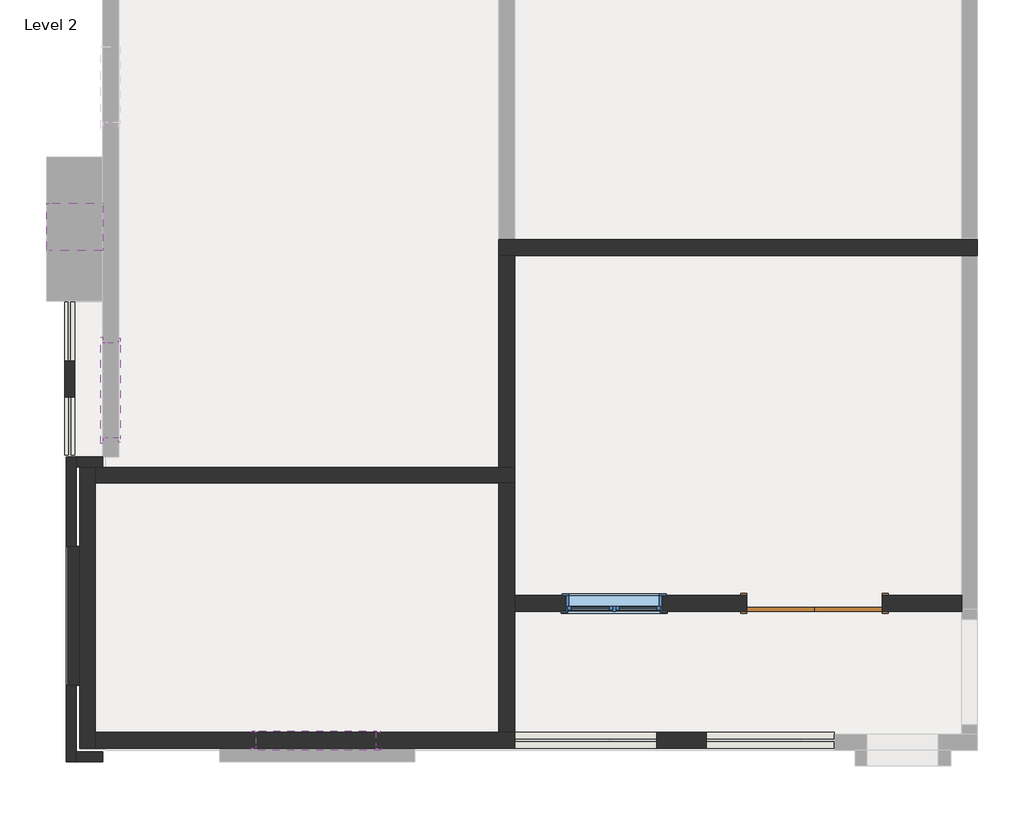
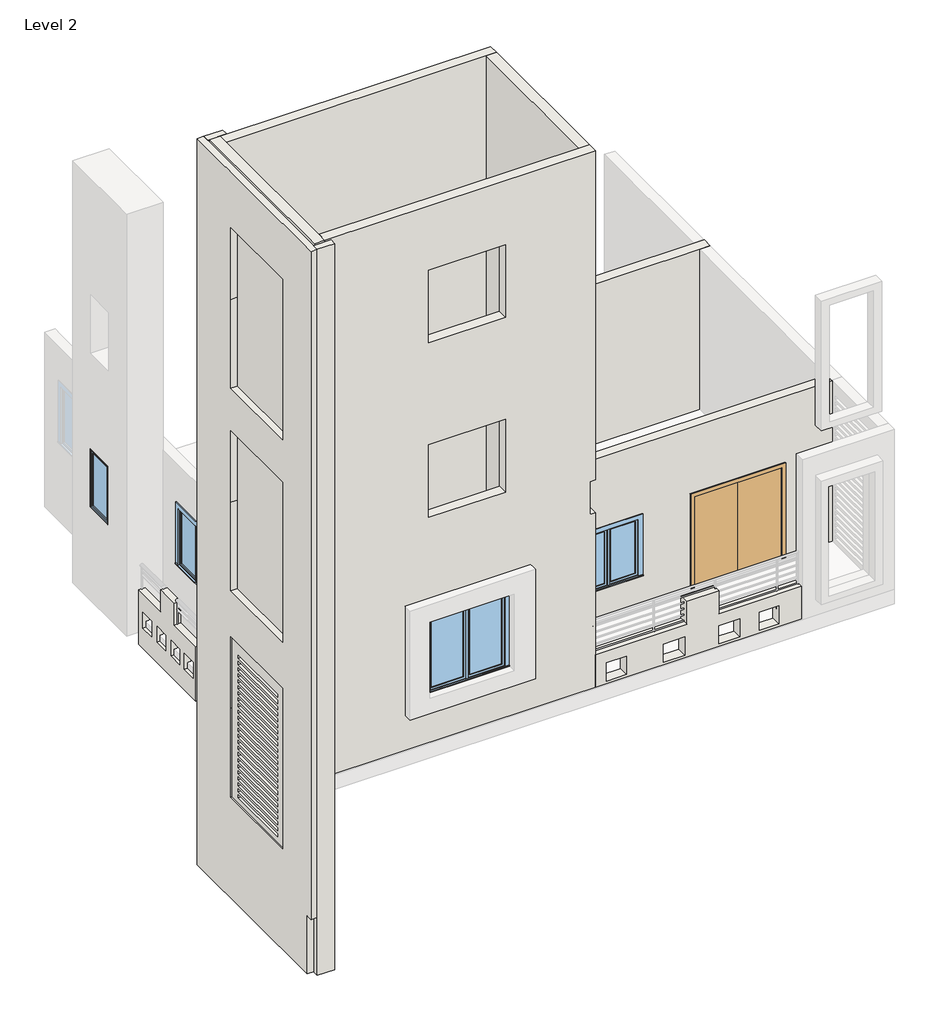
# One storey, part 1 of 2: 14 walls, 4 windows, 1 door.
"""IFC4 building model written with IfcOpenShell, lengths in millimetres."""

from ifc_helpers import new_model, si_unit, frame, origin, place, context, project, spatial, polyline, outline, extrude, faceted_brep, transform, mapped, element, save
from components import door_aae36eb6, window_0862ab64, window_514a67b1, window_df4b05bc

model = new_model("IFC4")

# Units and contexts
model_context = context("Model", 3, world=origin())
ifc_project = project(units=[si_unit("LENGTHUNIT", "METRE", prefix="MILLI")], contexts=[model_context])

# Site, building, storey
site = spatial("IfcSite", under=ifc_project)
building = spatial("IfcBuilding", under=site)
storey = spatial("IfcBuildingStorey", under=building, Name="Level 2", Elevation=3657.6)

# Door
placement = place(None, origin())
door_shape = door_aae36eb6(model_context)
element("IfcDoor", 1, ObjectType="Door-Double-Flush_Panel : 68\" x 80\"", at=placement, inside=storey, context=model_context, shape_type="MappedRepresentation", body=[
    mapped(door_shape, transform((-960.1997472, 3434.8484482, 3835.4), x_axis=(-1.0, 0.0, 0.0), y_axis=(0.0, -1.0, 0.0), z_axis=(0.0, 0.0, 1.0))),
])

# Walls
element("IfcWall", 2, ObjectType="Generic - 5\"", at=placement, inside=storey, context=model_context, shape_type="Brep", body=[
    faceted_brep([(-10524.0124309, 5306.9209854, 0.0), (-10524.0124309, 1535.0209854, 0.0), (-10524.0124309, 1535.0209854, 201.1297196), (-10524.0124309, 1535.0209854, 321.7975209), (-10524.0124309, 1535.0209854, 843.1993865), (-10524.0124309, 1535.0209854, 949.3856619), (-10524.0124309, 1535.0209854, 1213.0600738), (-10524.0124309, 1408.0209854, 1213.0600738), (-10524.0124309, 1408.0209854, 15198.970177), (-10524.0124309, 5306.9209854, 15198.970177), (-10524.0124309, 4162.4454783, 5461.9207805), (-10524.0124309, 2382.8579783, 5461.9207805), (-10524.0124309, 2382.8579783, 2106.7257577), (-10524.0124309, 4162.4454783, 2106.7257577), (-10524.0124309, 4162.4454783, 3962.4), (-10524.0124309, 4162.4454783, 9779.9207805), (-10524.0124309, 2382.8579783, 9779.9207805), (-10524.0124309, 2382.8579783, 6424.7257577), (-10524.0124309, 4162.4454783, 6424.7257577), (-10524.0124309, 4162.4454783, 8280.4), (-10524.0124309, 4162.4454783, 14023.1950228), (-10524.0124309, 2382.8579783, 14023.1950228), (-10524.0124309, 2382.8579783, 10668.0), (-10524.0124309, 4162.4454783, 10668.0), (-10524.0124309, 4162.4454783, 12523.6742423), (-10397.0124309, 5306.9209854, 0.0), (-10397.0124309, 5306.9209854, 15198.970177), (-10397.0124309, 5179.9209854, 15198.970177), (-10397.0124309, 1535.0209854, 15198.970177), (-10397.0124309, 1408.0209854, 15198.970177), (-10397.0124309, 1408.0209854, 1213.0600738), (-10397.0124309, 1535.0209854, 1213.0600738), (-10397.0124309, 1535.0209854, 0.0), (-10397.0124309, 5179.9209854, 0.0), (-10397.0124309, 4162.4454783, 5461.9207805), (-10397.0124309, 4162.4454783, 3962.4), (-10397.0124309, 4162.4454783, 2106.7257577), (-10397.0124309, 2382.8579783, 2106.7257577), (-10397.0124309, 2382.8579783, 5461.9207805), (-10397.0124309, 4162.4454783, 9779.9207805), (-10397.0124309, 4162.4454783, 8280.4), (-10397.0124309, 4162.4454783, 6424.7257577), (-10397.0124309, 2382.8579783, 6424.7257577), (-10397.0124309, 2382.8579783, 9779.9207805), (-10397.0124309, 4162.4454783, 14023.1950228), (-10397.0124309, 4162.4454783, 12523.6742423), (-10397.0124309, 4162.4454783, 10668.0), (-10397.0124309, 2382.8579783, 10668.0), (-10397.0124309, 2382.8579783, 14023.1950228), (-10502.5452839, 2382.8579783, 5461.9207805), (-10502.5452839, 2382.8579783, 2106.7257577)], [[[0, 1, 2, 3, 4, 5, 6, 7, 8, 9], [10, 11, 12, 13, 14], [15, 16, 17, 18, 19], [20, 21, 22, 23, 24]], [[25, 26, 27, 28, 29, 30, 31, 32, 33], [34, 35, 36, 37, 38], [39, 40, 41, 42, 43], [44, 45, 46, 47, 48]], [[0, 9, 26, 25]], [[1, 0, 25, 33, 32]], [[9, 8, 29, 28, 27, 26]], [[10, 14, 35, 34]], [[11, 49, 38, 37, 50, 12]], [[13, 12, 50, 37, 36]], [[14, 13, 36, 35]], [[11, 10, 34, 38, 49]], [[16, 15, 39, 43]], [[18, 17, 42, 41]], [[19, 18, 41, 40]], [[15, 19, 40, 39]], [[21, 20, 44, 48]], [[23, 22, 47, 46]], [[24, 23, 46, 45]], [[20, 24, 45, 44]], [[16, 43, 42, 17]], [[21, 48, 47, 22]], [[30, 7, 6, 31]], [[1, 32, 31, 6, 5, 4, 3, 2]], [[8, 7, 30, 29]]]),
])
element("IfcWall", 3, ObjectType="Generic - 5\"", at=placement, inside=storey, context=model_context, shape_type="SweptSolid", body=[
    extrude(outline(polyline([(0.0, -10397.0124309), (0.0, -10053.3997472), (11277.6, -10053.3997472), (11277.6, -10018.4747472), (15198.970177, -10018.4747472), (15198.970177, -10397.0124309), (0.0, -10397.0124309)])), frame((0.0, 5179.9209854, 0.0), z_axis=(0.0, 1.0, 0.0), x_axis=(0.0, 0.0, 1.0)), (0.0, 0.0, 1.0), 127.0),
])
element("IfcWall", 4, ObjectType="Generic - 5\"", at=placement, inside=storey, context=model_context, shape_type="Brep", body=[
    faceted_brep([(-10397.0124309, 1408.0209854, 15198.970177), (-10397.0124309, 1408.0209854, 1213.0600738), (-10397.0124309, 1408.0209854, 0.0), (-10053.3997472, 1408.0209854, 0.0), (-10053.3997472, 1408.0209854, 15198.970177), (-10397.0124309, 1535.0209854, 0.0), (-10397.0124309, 1535.0209854, 1213.0600738), (-10397.0124309, 1535.0209854, 15198.970177), (-10053.3997472, 1535.0209854, 15198.970177), (-10053.3997472, 1535.0209854, 0.0)], [[[0, 1, 2, 3, 4]], [[5, 6, 7, 8, 9]], [[3, 2, 5, 9]], [[0, 4, 8, 7]], [[4, 3, 9, 8]], [[0, 7, 6, 5, 2, 1]]]),
])
element("IfcWall", 5, ObjectType="Generic - 5\"", at=placement, inside=storey, context=model_context, shape_type="SweptSolid", body=[
    extrude(outline(polyline([(7286.192958, 3413.4386364), (5330.392958, 3413.4386364), (5330.392958, 4554.6632192), (6074.2144874, 4554.6632192), (6074.2144874, 5011.8632192), (6531.4144874, 5011.8632192), (6531.4144874, 4554.6632192), (7286.192958, 4554.6632192), (7286.192958, 3413.4386364)]), holes=[polyline([(6843.8232349, 4170.3459623), (6843.8232349, 3840.1459623), (7148.6232349, 3840.1459623), (7148.6232349, 4170.3459623), (6843.8232349, 4170.3459623)]), polyline([(6361.2232349, 4170.3459623), (6361.2232349, 3840.1459623), (6666.0232349, 3840.1459623), (6666.0232349, 4170.3459623), (6361.2232349, 4170.3459623)]), polyline([(5878.6232349, 4170.3459623), (5878.6232349, 3840.1459623), (6183.4232349, 3840.1459623), (6183.4232349, 4170.3459623), (5878.6232349, 4170.3459623)]), polyline([(5421.4232349, 4170.3459623), (5421.4232349, 3840.1459623), (5726.2232349, 3840.1459623), (5726.2232349, 4170.3459623), (5421.4232349, 4170.3459623)])]), frame((-10539.1747472, 0.0, 0.0), z_axis=(1.0, 0.0, 0.0), x_axis=(0.0, 1.0, 0.0)), (0.0, 0.0, 1.0), 127.0),
])
element("IfcWall", 6, ObjectType="Generic - 8\"", at=placement, inside=storey, context=model_context, shape_type="Brep", body=[
    faceted_brep([(-10149.3857575, 1580.6484482, 3657.6), (-10149.3857575, 1783.8484482, 3657.6), (-10149.3857575, 4971.5484482, 3657.6), (-10149.3857575, 5174.7484482, 3657.6), (-10149.3857575, 5174.7484482, 15198.970177), (-10149.3857575, 4971.5484482, 15198.970177), (-10149.3857575, 1580.6484482, 15198.970177), (-10352.5857575, 1580.6484482, 3657.6), (-10352.5857575, 1580.6484482, 15198.970177), (-10352.5857575, 5174.7484482, 15198.970177), (-10352.5857575, 5174.7484482, 3657.6)], [[[0, 1, 2, 3, 4, 5, 6]], [[7, 8, 9, 10]], [[3, 2, 1, 0, 7, 10]], [[6, 5, 4, 9, 8]], [[0, 6, 8, 7]], [[4, 3, 10, 9]]]),
])
element("IfcWall", 7, ObjectType="Generic - 8\"", at=placement, inside=storey, context=model_context, shape_type="Brep", body=[
    faceted_brep([(-10149.3857575, 4971.5484482, 3657.6), (-4993.1857575, 4971.5484482, 3657.6), (-4789.9857575, 4971.5484482, 3657.6), (-4789.9857575, 4971.5484482, 15198.970177), (-4993.1857575, 4971.5484482, 15198.970177), (-10149.3857575, 4971.5484482, 15198.970177), (-10149.3857575, 5174.7484482, 3657.6), (-10149.3857575, 5174.7484482, 15198.970177), (-4789.9857575, 5174.7484482, 15198.970177), (-4789.9857575, 5174.7484482, 10972.8), (-4789.9857575, 5174.7484482, 7315.2), (-4789.9857575, 5174.7484482, 3657.6), (-4993.1857575, 5174.7484482, 3657.6)], [[[0, 1, 2, 3, 4, 5]], [[6, 7, 8, 9, 10, 11, 12]], [[2, 1, 0, 6, 12, 11]], [[5, 4, 3, 8, 7]], [[0, 5, 7, 6]], [[2, 11, 10, 9, 8, 3]]]),
])
element("IfcWall", 8, ObjectType="Generic - 8\"", at=placement, inside=storey, context=model_context, shape_type="Brep", body=[
    faceted_brep([(-10149.3857575, 1580.6484482, 3657.6), (-4789.9857575, 1580.6484482, 3657.6), (-4789.9857575, 1580.6484482, 3962.4), (-4789.9857575, 1580.6484482, 4648.2), (-4789.9857575, 1580.6484482, 7620.0), (-4891.5857575, 1580.6484482, 7620.0), (-4891.5857575, 1580.6484482, 8305.8), (-4789.9857575, 1580.6484482, 8305.8), (-4789.9857575, 1580.6484482, 15201.7585229), (-10149.3857575, 1580.6484482, 15201.7585229), (-10149.3857575, 1580.6484482, 15198.970177), (-8091.9857575, 1580.6484482, 6540.6181256), (-6567.9857575, 1580.6484482, 6540.6181256), (-6567.9857575, 1580.6484482, 5016.6181256), (-8091.9857575, 1580.6484482, 5016.6181256), (-8091.9857575, 1580.6484482, 10198.2181256), (-6567.9857575, 1580.6484482, 10198.2181256), (-6567.9857575, 1580.6484482, 8674.2181256), (-8091.9857575, 1580.6484482, 8674.2181256), (-8091.9857575, 1580.6484482, 13855.8181256), (-6567.9857575, 1580.6484482, 13855.8181256), (-6567.9857575, 1580.6484482, 12331.8181256), (-8091.9857575, 1580.6484482, 12331.8181256), (-10149.3857575, 1783.8484482, 3657.6), (-10149.3857575, 1783.8484482, 15201.7585229), (-4789.9857575, 1783.8484482, 15201.7585229), (-4789.9857575, 1783.8484482, 15198.970177), (-4789.9857575, 1783.8484482, 8305.8), (-4891.5857575, 1783.8484482, 8305.8), (-4891.5857575, 1783.8484482, 7620.0), (-4789.9857575, 1783.8484482, 7620.0), (-4789.9857575, 1783.8484482, 4648.2), (-4789.9857575, 1783.8484482, 3962.4), (-4789.9857575, 1783.8484482, 3657.6), (-4993.1857575, 1783.8484482, 3657.6), (-8091.9857575, 1783.8484482, 6540.6181256), (-8091.9857575, 1783.8484482, 5016.6181256), (-6567.9857575, 1783.8484482, 5016.6181256), (-6567.9857575, 1783.8484482, 6540.6181256), (-8091.9857575, 1783.8484482, 10198.2181256), (-8091.9857575, 1783.8484482, 8674.2181256), (-6567.9857575, 1783.8484482, 8674.2181256), (-6567.9857575, 1783.8484482, 10198.2181256), (-8091.9857575, 1783.8484482, 13855.8181256), (-8091.9857575, 1783.8484482, 12331.8181256), (-6567.9857575, 1783.8484482, 12331.8181256), (-6567.9857575, 1783.8484482, 13855.8181256)], [[[0, 1, 2, 3, 4, 5, 6, 7, 8, 9, 10], [11, 12, 13, 14], [15, 16, 17, 18], [19, 20, 21, 22]], [[23, 24, 25, 26, 27, 28, 29, 30, 31, 32, 33, 34], [35, 36, 37, 38], [39, 40, 41, 42], [43, 44, 45, 46]], [[1, 0, 23, 34, 33]], [[9, 8, 25, 24]], [[0, 10, 9, 24, 23]], [[36, 35, 11, 14]], [[37, 36, 14, 13]], [[38, 37, 13, 12]], [[35, 38, 12, 11]], [[40, 39, 15, 18]], [[41, 40, 18, 17]], [[42, 41, 17, 16]], [[39, 42, 16, 15]], [[44, 43, 19, 22]], [[45, 44, 22, 21]], [[46, 45, 21, 20]], [[43, 46, 20, 19]], [[29, 5, 4, 30]], [[5, 29, 28, 6]], [[27, 7, 6, 28]], [[1, 33, 32, 31, 30, 4, 3, 2]], [[8, 7, 27, 26, 25]]]),
])
element("IfcWall", 9, ObjectType="Generic - 8\"", at=placement, inside=storey, context=model_context, shape_type="Brep", body=[
    faceted_brep([(-4993.1857575, 4971.5484482, 15198.970177), (-4993.1857575, 4971.5484482, 3657.6), (-4993.1857575, 1783.8484482, 3657.6), (-4993.1857575, 1783.8484482, 15198.970177), (-4789.9857575, 4971.5484482, 3657.6), (-4789.9857575, 4971.5484482, 15198.970177), (-4789.9857575, 1783.8484482, 15198.970177), (-4789.9857575, 1783.8484482, 8305.8), (-4789.9857575, 1783.8484482, 7620.0), (-4789.9857575, 1783.8484482, 3657.6), (-4789.9857575, 3333.2484482, 3657.6), (-4789.9857575, 3536.4484482, 3657.6)], [[[0, 1, 2, 3]], [[4, 5, 6, 7, 8, 9, 10, 11]], [[2, 1, 4, 11, 10, 9]], [[0, 3, 6, 5]], [[0, 5, 4, 1]], [[2, 9, 8, 7, 6, 3]]]),
])
element("IfcWall", 10, ObjectType="Generic - 8\"", at=placement, inside=storey, context=model_context, shape_type="Brep", body=[
    faceted_brep([(-4789.9857575, 3333.2484482, 3657.6), (919.4002528, 3333.2484482, 3657.6), (919.4002528, 3333.2484482, 3962.4), (919.4002528, 3333.2484482, 7315.2), (-4789.9857575, 3333.2484482, 7315.2), (-1823.7997472, 3333.2484482, 3835.4), (-1823.7997472, 3333.2484482, 5867.4), (-96.5997472, 3333.2484482, 5867.4), (-96.5997472, 3333.2484482, 3835.4), (-4129.5857575, 3333.2484482, 4572.0), (-4129.5857575, 3333.2484482, 5791.2), (-2910.3857575, 3333.2484482, 5791.2), (-2910.3857575, 3333.2484482, 4572.0), (919.4002528, 3536.4484482, 3657.6), (-4789.9857575, 3536.4484482, 3657.6), (-4789.9857575, 3536.4484482, 7315.2), (919.4002528, 3536.4484482, 7315.2), (-1823.7997472, 3536.4484482, 5867.4), (-1823.7997472, 3536.4484482, 3835.4), (-96.5997472, 3536.4484482, 3835.4), (-96.5997472, 3536.4484482, 5867.4), (-4129.5857575, 3536.4484482, 5791.2), (-4129.5857575, 3536.4484482, 4572.0), (-2910.3857575, 3536.4484482, 4572.0), (-2910.3857575, 3536.4484482, 5791.2), (919.4002528, 3358.6484482, 7315.2)], [[[0, 1, 2, 3, 4], [5, 6, 7, 8], [9, 10, 11, 12]], [[13, 14, 15, 16], [17, 18, 19, 20], [21, 22, 23, 24]], [[1, 0, 14, 13]], [[4, 3, 25, 16, 15]], [[0, 4, 15, 14]], [[1, 13, 16, 25, 3, 2]], [[5, 18, 17, 6]], [[6, 17, 20, 7]], [[7, 20, 19, 8]], [[18, 5, 8, 19]], [[22, 21, 10, 9]], [[23, 22, 9, 12]], [[24, 23, 12, 11]], [[21, 24, 11, 10]]]),
])
element("IfcWall", 11, ObjectType="Generic - 8\"", at=placement, inside=storey, context=model_context, shape_type="Brep", body=[
    faceted_brep([(1122.6002528, 8083.0484482, 3657.6), (-4789.9857575, 8083.0484482, 3657.6), (-4993.1857575, 8083.0484482, 3657.6), (-4993.1857575, 8083.0484482, 7315.2), (-4789.9857575, 8083.0484482, 7315.2), (1122.6002528, 8083.0484482, 7315.2), (1122.6002528, 7879.8484482, 3657.6), (1122.6002528, 7879.8484482, 7315.2), (919.4002528, 7879.8484482, 7315.2), (-4789.9857575, 7879.8484482, 7315.2), (-4993.1857575, 7879.8484482, 7315.2), (-4993.1857575, 7879.8484482, 3657.6), (-4789.9857575, 7879.8484482, 3657.6), (919.4002528, 7879.8484482, 3657.6)], [[[0, 1, 2, 3, 4, 5]], [[6, 7, 8, 9, 10, 11, 12, 13]], [[2, 1, 0, 6, 13, 12, 11]], [[5, 4, 3, 10, 9, 8, 7]], [[3, 2, 11, 10]], [[0, 5, 7, 6]]]),
])
element("IfcWall", 12, ObjectType="Generic - 8\"", at=placement, inside=storey, context=model_context, shape_type="SweptSolid", body=[
    extrude(outline(polyline([(-4993.1857575, 5174.7484482), (-4993.1857575, 7879.8484482), (-4789.9857575, 7879.8484482), (-4789.9857575, 5174.7484482), (-4993.1857575, 5174.7484482)])), frame((0.0, 0.0, 3657.6), z_axis=(0.0, 0.0, 1.0), x_axis=(1.0, 0.0, 0.0)), (0.0, 0.0, 1.0), 3657.6),
])
element("IfcWall", 13, ObjectType="Generic - 8\"", at=placement, inside=storey, context=model_context, shape_type="SweptSolid", body=[
    extrude(outline(polyline([(3962.4, -4789.9857575), (3962.4, -706.1997472), (4648.2, -706.1997472), (4648.2, -2342.0957574), (5130.8, -2342.0957574), (5130.8, -2973.8857575), (4648.2, -2973.8857575), (4648.2, -4789.9857575), (3962.4, -4789.9857575)]), holes=[polyline([(4395.9967121, -4172.8537192), (4014.9967121, -4172.8537192), (4014.9967121, -4568.8757796), (4395.9967121, -4568.8757796), (4395.9967121, -4172.8537192)]), polyline([(4395.9967121, -3016.3977147), (4014.9967121, -3016.3977147), (4014.9967121, -3442.485742), (4395.9967121, -3442.485742), (4395.9967121, -3016.3977147)]), polyline([(4395.9967121, -1925.4048959), (4014.9967121, -1925.4048959), (4014.9967121, -2342.0957574), (4395.9967121, -2342.0957574), (4395.9967121, -1925.4048959)]), polyline([(4395.9967121, -1149.8086357), (4014.9967121, -1149.8086357), (4014.9967121, -1533.9667029), (4395.9967121, -1533.9667029), (4395.9967121, -1149.8086357)])]), frame((0.0, 1580.6484482, 0.0), z_axis=(0.0, 1.0, 0.0), x_axis=(0.0, 0.0, 1.0)), (0.0, 0.0, 1.0), 203.2),
])
element("IfcWall", 14, ObjectType="Generic - 8\"", at=placement, inside=storey, context=model_context, shape_type="Brep", body=[
    faceted_brep([(-10299.3452839, 4162.4454783, 2106.7257577), (-10299.3452839, 4162.4454783, 5461.9207805), (-10299.3452839, 2382.8579783, 5461.9207805), (-10299.3452839, 2382.8579783, 2106.7257577), (-10299.3452839, 3937.4533381, 5200.9799759), (-10299.3452839, 3937.4533381, 5137.4799759), (-10299.3452839, 2591.2533381, 5137.4799759), (-10299.3452839, 2591.2533381, 5200.9799759), (-10299.3452839, 3937.4533381, 5073.9799759), (-10299.3452839, 3937.4533381, 5010.4799759), (-10299.3452839, 2591.2533381, 5010.4799759), (-10299.3452839, 2591.2533381, 5073.9799759), (-10299.3452839, 3937.4533381, 4946.9799759), (-10299.3452839, 3937.4533381, 4883.4799759), (-10299.3452839, 2591.2533381, 4883.4799759), (-10299.3452839, 2591.2533381, 4946.9799759), (-10299.3452839, 3937.4533381, 4819.9799759), (-10299.3452839, 3937.4533381, 4756.4799759), (-10299.3452839, 2591.2533381, 4756.4799759), (-10299.3452839, 2591.2533381, 4819.9799759), (-10299.3452839, 3937.4533381, 4692.9799759), (-10299.3452839, 3937.4533381, 4629.4799759), (-10299.3452839, 2591.2533381, 4629.4799759), (-10299.3452839, 2591.2533381, 4692.9799759), (-10299.3452839, 3937.4533381, 4565.9799759), (-10299.3452839, 3937.4533381, 4502.4799759), (-10299.3452839, 2591.2533381, 4502.4799759), (-10299.3452839, 2591.2533381, 4565.9799759), (-10299.3452839, 3937.4533381, 4438.9799759), (-10299.3452839, 3937.4533381, 4375.4799759), (-10299.3452839, 2591.2533381, 4375.4799759), (-10299.3452839, 2591.2533381, 4438.9799759), (-10299.3452839, 3937.4533381, 4311.9799759), (-10299.3452839, 3937.4533381, 4248.4799759), (-10299.3452839, 2591.2533381, 4248.4799759), (-10299.3452839, 2591.2533381, 4311.9799759), (-10299.3452839, 3937.4533381, 4184.9799759), (-10299.3452839, 3937.4533381, 4121.4799759), (-10299.3452839, 2591.2533381, 4121.4799759), (-10299.3452839, 2591.2533381, 4184.9799759), (-10299.3452839, 3937.4533381, 4057.9799759), (-10299.3452839, 3937.4533381, 3994.4799759), (-10299.3452839, 2591.2533381, 3994.4799759), (-10299.3452839, 2591.2533381, 4057.9799759), (-10299.3452839, 3937.4533381, 3930.9799759), (-10299.3452839, 3937.4533381, 3867.4799759), (-10299.3452839, 2591.2533381, 3867.4799759), (-10299.3452839, 2591.2533381, 3930.9799759), (-10299.3452839, 3937.4533381, 3803.9799759), (-10299.3452839, 3937.4533381, 3740.4799759), (-10299.3452839, 2591.2533381, 3740.4799759), (-10299.3452839, 2591.2533381, 3803.9799759), (-10299.3452839, 3937.4533381, 3676.9799759), (-10299.3452839, 3937.4533381, 3613.4799759), (-10299.3452839, 2591.2533381, 3613.4799759), (-10299.3452839, 2591.2533381, 3676.9799759), (-10299.3452839, 3937.4533381, 3549.9799759), (-10299.3452839, 3937.4533381, 3486.4799759), (-10299.3452839, 2591.2533381, 3486.4799759), (-10299.3452839, 2591.2533381, 3549.9799759), (-10299.3452839, 3937.4533381, 3422.9799759), (-10299.3452839, 3937.4533381, 3359.4799759), (-10299.3452839, 2591.2533381, 3359.4799759), (-10299.3452839, 2591.2533381, 3422.9799759), (-10299.3452839, 3937.4533381, 3295.9799759), (-10299.3452839, 3937.4533381, 3232.4799759), (-10299.3452839, 2591.2533381, 3232.4799759), (-10299.3452839, 2591.2533381, 3295.9799759), (-10299.3452839, 3937.4533381, 3168.9799759), (-10299.3452839, 3937.4533381, 3105.4799759), (-10299.3452839, 2591.2533381, 3105.4799759), (-10299.3452839, 2591.2533381, 3168.9799759), (-10299.3452839, 3937.4533381, 3041.9799759), (-10299.3452839, 3937.4533381, 2978.4799759), (-10299.3452839, 2591.2533381, 2978.4799759), (-10299.3452839, 2591.2533381, 3041.9799759), (-10299.3452839, 3937.4533381, 2914.9799759), (-10299.3452839, 3937.4533381, 2851.4799759), (-10299.3452839, 2591.2533381, 2851.4799759), (-10299.3452839, 2591.2533381, 2914.9799759), (-10299.3452839, 3937.4533381, 2787.9799759), (-10299.3452839, 3937.4533381, 2724.4799759), (-10299.3452839, 2591.2533381, 2724.4799759), (-10299.3452839, 2591.2533381, 2787.9799759), (-10299.3452839, 3937.4533381, 2660.9799759), (-10299.3452839, 3937.4533381, 2597.4799759), (-10299.3452839, 2591.2533381, 2597.4799759), (-10299.3452839, 2591.2533381, 2660.9799759), (-10299.3452839, 3937.4533381, 2533.9799759), (-10299.3452839, 3937.4533381, 2470.4799759), (-10299.3452839, 2591.2533381, 2470.4799759), (-10299.3452839, 2591.2533381, 2533.9799759), (-10299.3452839, 3937.4533381, 2406.9799759), (-10299.3452839, 3937.4533381, 2343.4799759), (-10299.3452839, 2591.2533381, 2343.4799759), (-10299.3452839, 2591.2533381, 2406.9799759), (-10299.3452839, 3937.4533381, 2279.9799759), (-10299.3452839, 3937.4533381, 2216.4799759), (-10299.3452839, 2591.2533381, 2216.4799759), (-10299.3452839, 2591.2533381, 2279.9799759), (-10502.5452839, 4162.4454783, 2106.7257577), (-10502.5452839, 2382.8579783, 2106.7257577), (-10502.5452839, 2382.8579783, 5461.9207805), (-10502.5452839, 4162.4454783, 5461.9207805), (-10502.5452839, 3937.4533381, 5200.9799759), (-10502.5452839, 2591.2533381, 5200.9799759), (-10502.5452839, 2591.2533381, 5137.4799759), (-10502.5452839, 3937.4533381, 5137.4799759), (-10502.5452839, 3937.4533381, 5073.9799759), (-10502.5452839, 2591.2533381, 5073.9799759), (-10502.5452839, 2591.2533381, 5010.4799759), (-10502.5452839, 3937.4533381, 5010.4799759), (-10502.5452839, 3937.4533381, 4946.9799759), (-10502.5452839, 2591.2533381, 4946.9799759), (-10502.5452839, 2591.2533381, 4883.4799759), (-10502.5452839, 3937.4533381, 4883.4799759), (-10502.5452839, 3937.4533381, 4819.9799759), (-10502.5452839, 2591.2533381, 4819.9799759), (-10502.5452839, 2591.2533381, 4756.4799759), (-10502.5452839, 3937.4533381, 4756.4799759), (-10502.5452839, 3937.4533381, 4692.9799759), (-10502.5452839, 2591.2533381, 4692.9799759), (-10502.5452839, 2591.2533381, 4629.4799759), (-10502.5452839, 3937.4533381, 4629.4799759), (-10502.5452839, 3937.4533381, 4565.9799759), (-10502.5452839, 2591.2533381, 4565.9799759), (-10502.5452839, 2591.2533381, 4502.4799759), (-10502.5452839, 3937.4533381, 4502.4799759), (-10502.5452839, 3937.4533381, 4438.9799759), (-10502.5452839, 2591.2533381, 4438.9799759), (-10502.5452839, 2591.2533381, 4375.4799759), (-10502.5452839, 3937.4533381, 4375.4799759), (-10502.5452839, 3937.4533381, 4311.9799759), (-10502.5452839, 2591.2533381, 4311.9799759), (-10502.5452839, 2591.2533381, 4248.4799759), (-10502.5452839, 3937.4533381, 4248.4799759), (-10502.5452839, 3937.4533381, 4184.9799759), (-10502.5452839, 2591.2533381, 4184.9799759), (-10502.5452839, 2591.2533381, 4121.4799759), (-10502.5452839, 3937.4533381, 4121.4799759), (-10502.5452839, 3937.4533381, 4057.9799759), (-10502.5452839, 2591.2533381, 4057.9799759), (-10502.5452839, 2591.2533381, 3994.4799759), (-10502.5452839, 3937.4533381, 3994.4799759), (-10502.5452839, 3937.4533381, 3930.9799759), (-10502.5452839, 2591.2533381, 3930.9799759), (-10502.5452839, 2591.2533381, 3867.4799759), (-10502.5452839, 3937.4533381, 3867.4799759), (-10502.5452839, 3937.4533381, 3803.9799759), (-10502.5452839, 2591.2533381, 3803.9799759), (-10502.5452839, 2591.2533381, 3740.4799759), (-10502.5452839, 3937.4533381, 3740.4799759), (-10502.5452839, 3937.4533381, 3676.9799759), (-10502.5452839, 2591.2533381, 3676.9799759), (-10502.5452839, 2591.2533381, 3613.4799759), (-10502.5452839, 3937.4533381, 3613.4799759), (-10502.5452839, 3937.4533381, 3549.9799759), (-10502.5452839, 2591.2533381, 3549.9799759), (-10502.5452839, 2591.2533381, 3486.4799759), (-10502.5452839, 3937.4533381, 3486.4799759), (-10502.5452839, 3937.4533381, 3422.9799759), (-10502.5452839, 2591.2533381, 3422.9799759), (-10502.5452839, 2591.2533381, 3359.4799759), (-10502.5452839, 3937.4533381, 3359.4799759), (-10502.5452839, 3937.4533381, 3295.9799759), (-10502.5452839, 2591.2533381, 3295.9799759), (-10502.5452839, 2591.2533381, 3232.4799759), (-10502.5452839, 3937.4533381, 3232.4799759), (-10502.5452839, 3937.4533381, 3168.9799759), (-10502.5452839, 2591.2533381, 3168.9799759), (-10502.5452839, 2591.2533381, 3105.4799759), (-10502.5452839, 3937.4533381, 3105.4799759), (-10502.5452839, 3937.4533381, 3041.9799759), (-10502.5452839, 2591.2533381, 3041.9799759), (-10502.5452839, 2591.2533381, 2978.4799759), (-10502.5452839, 3937.4533381, 2978.4799759), (-10502.5452839, 3937.4533381, 2914.9799759), (-10502.5452839, 2591.2533381, 2914.9799759), (-10502.5452839, 2591.2533381, 2851.4799759), (-10502.5452839, 3937.4533381, 2851.4799759), (-10502.5452839, 3937.4533381, 2787.9799759), (-10502.5452839, 2591.2533381, 2787.9799759), (-10502.5452839, 2591.2533381, 2724.4799759), (-10502.5452839, 3937.4533381, 2724.4799759), (-10502.5452839, 3937.4533381, 2660.9799759), (-10502.5452839, 2591.2533381, 2660.9799759), (-10502.5452839, 2591.2533381, 2597.4799759), (-10502.5452839, 3937.4533381, 2597.4799759), (-10502.5452839, 3937.4533381, 2533.9799759), (-10502.5452839, 2591.2533381, 2533.9799759), (-10502.5452839, 2591.2533381, 2470.4799759), (-10502.5452839, 3937.4533381, 2470.4799759), (-10502.5452839, 3937.4533381, 2406.9799759), (-10502.5452839, 2591.2533381, 2406.9799759), (-10502.5452839, 2591.2533381, 2343.4799759), (-10502.5452839, 3937.4533381, 2343.4799759), (-10502.5452839, 3937.4533381, 2279.9799759), (-10502.5452839, 2591.2533381, 2279.9799759), (-10502.5452839, 2591.2533381, 2216.4799759), (-10502.5452839, 3937.4533381, 2216.4799759), (-10397.0124309, 2382.8579783, 2106.7257577), (-10397.0124309, 2382.8579783, 5461.9207805)], [[[0, 1, 2, 3], [4, 5, 6, 7], [8, 9, 10, 11], [12, 13, 14, 15], [16, 17, 18, 19], [20, 21, 22, 23], [24, 25, 26, 27], [28, 29, 30, 31], [32, 33, 34, 35], [36, 37, 38, 39], [40, 41, 42, 43], [44, 45, 46, 47], [48, 49, 50, 51], [52, 53, 54, 55], [56, 57, 58, 59], [60, 61, 62, 63], [64, 65, 66, 67], [68, 69, 70, 71], [72, 73, 74, 75], [76, 77, 78, 79], [80, 81, 82, 83], [84, 85, 86, 87], [88, 89, 90, 91], [92, 93, 94, 95], [96, 97, 98, 99]], [[100, 101, 102, 103], [104, 105, 106, 107], [108, 109, 110, 111], [112, 113, 114, 115], [116, 117, 118, 119], [120, 121, 122, 123], [124, 125, 126, 127], [128, 129, 130, 131], [132, 133, 134, 135], [136, 137, 138, 139], [140, 141, 142, 143], [144, 145, 146, 147], [148, 149, 150, 151], [152, 153, 154, 155], [156, 157, 158, 159], [160, 161, 162, 163], [164, 165, 166, 167], [168, 169, 170, 171], [172, 173, 174, 175], [176, 177, 178, 179], [180, 181, 182, 183], [184, 185, 186, 187], [188, 189, 190, 191], [192, 193, 194, 195], [196, 197, 198, 199]], [[0, 3, 200, 101, 100]], [[2, 1, 103, 102, 201]], [[1, 0, 100, 103]], [[5, 4, 104, 107]], [[6, 5, 107, 106]], [[7, 6, 106, 105]], [[4, 7, 105, 104]], [[9, 8, 108, 111]], [[10, 9, 111, 110]], [[11, 10, 110, 109]], [[8, 11, 109, 108]], [[13, 12, 112, 115]], [[14, 13, 115, 114]], [[15, 14, 114, 113]], [[12, 15, 113, 112]], [[17, 16, 116, 119]], [[18, 17, 119, 118]], [[19, 18, 118, 117]], [[16, 19, 117, 116]], [[21, 20, 120, 123]], [[22, 21, 123, 122]], [[23, 22, 122, 121]], [[20, 23, 121, 120]], [[25, 24, 124, 127]], [[26, 25, 127, 126]], [[27, 26, 126, 125]], [[24, 27, 125, 124]], [[29, 28, 128, 131]], [[30, 29, 131, 130]], [[31, 30, 130, 129]], [[28, 31, 129, 128]], [[33, 32, 132, 135]], [[34, 33, 135, 134]], [[35, 34, 134, 133]], [[32, 35, 133, 132]], [[37, 36, 136, 139]], [[38, 37, 139, 138]], [[39, 38, 138, 137]], [[36, 39, 137, 136]], [[41, 40, 140, 143]], [[42, 41, 143, 142]], [[43, 42, 142, 141]], [[40, 43, 141, 140]], [[45, 44, 144, 147]], [[46, 45, 147, 146]], [[47, 46, 146, 145]], [[44, 47, 145, 144]], [[49, 48, 148, 151]], [[50, 49, 151, 150]], [[51, 50, 150, 149]], [[48, 51, 149, 148]], [[53, 52, 152, 155]], [[54, 53, 155, 154]], [[55, 54, 154, 153]], [[52, 55, 153, 152]], [[57, 56, 156, 159]], [[58, 57, 159, 158]], [[59, 58, 158, 157]], [[56, 59, 157, 156]], [[61, 60, 160, 163]], [[62, 61, 163, 162]], [[63, 62, 162, 161]], [[60, 63, 161, 160]], [[65, 64, 164, 167]], [[66, 65, 167, 166]], [[67, 66, 166, 165]], [[64, 67, 165, 164]], [[69, 68, 168, 171]], [[70, 69, 171, 170]], [[71, 70, 170, 169]], [[68, 71, 169, 168]], [[73, 72, 172, 175]], [[74, 73, 175, 174]], [[75, 74, 174, 173]], [[72, 75, 173, 172]], [[77, 76, 176, 179]], [[78, 77, 179, 178]], [[79, 78, 178, 177]], [[76, 79, 177, 176]], [[81, 80, 180, 183]], [[82, 81, 183, 182]], [[83, 82, 182, 181]], [[80, 83, 181, 180]], [[85, 84, 184, 187]], [[86, 85, 187, 186]], [[87, 86, 186, 185]], [[84, 87, 185, 184]], [[89, 88, 188, 191]], [[90, 89, 191, 190]], [[91, 90, 190, 189]], [[88, 91, 189, 188]], [[93, 92, 192, 195]], [[94, 93, 195, 194]], [[95, 94, 194, 193]], [[92, 95, 193, 192]], [[97, 96, 196, 199]], [[98, 97, 199, 198]], [[99, 98, 198, 197]], [[96, 99, 197, 196]], [[2, 201, 102, 101, 200, 3]]]),
])
element("IfcWall", 15, ObjectType="Generic - 8\"", at=placement, inside=storey, context=model_context, shape_type="SweptSolid", body=[
    extrude(outline(polyline([(4162.4454783, 2106.7257577), (2382.8579783, 2106.7257577), (2382.8579783, 5461.9207805), (4162.4454783, 5461.9207805), (4162.4454783, 2106.7257577)]), holes=[polyline([(3937.4533381, 5200.9799759), (2591.2533381, 5200.9799759), (2591.2533381, 5137.4799759), (3937.4533381, 5137.4799759), (3937.4533381, 5200.9799759)]), polyline([(3937.4533381, 5073.9799759), (2591.2533381, 5073.9799759), (2591.2533381, 5010.4799759), (3937.4533381, 5010.4799759), (3937.4533381, 5073.9799759)]), polyline([(3937.4533381, 4946.9799759), (2591.2533381, 4946.9799759), (2591.2533381, 4883.4799759), (3937.4533381, 4883.4799759), (3937.4533381, 4946.9799759)]), polyline([(3937.4533381, 4819.9799759), (2591.2533381, 4819.9799759), (2591.2533381, 4756.4799759), (3937.4533381, 4756.4799759), (3937.4533381, 4819.9799759)]), polyline([(3937.4533381, 4692.9799759), (2591.2533381, 4692.9799759), (2591.2533381, 4629.4799759), (3937.4533381, 4629.4799759), (3937.4533381, 4692.9799759)]), polyline([(3937.4533381, 4565.9799759), (2591.2533381, 4565.9799759), (2591.2533381, 4502.4799759), (3937.4533381, 4502.4799759), (3937.4533381, 4565.9799759)]), polyline([(3937.4533381, 4438.9799759), (2591.2533381, 4438.9799759), (2591.2533381, 4375.4799759), (3937.4533381, 4375.4799759), (3937.4533381, 4438.9799759)]), polyline([(3937.4533381, 4311.9799759), (2591.2533381, 4311.9799759), (2591.2533381, 4248.4799759), (3937.4533381, 4248.4799759), (3937.4533381, 4311.9799759)]), polyline([(3937.4533381, 4184.9799759), (2591.2533381, 4184.9799759), (2591.2533381, 4121.4799759), (3937.4533381, 4121.4799759), (3937.4533381, 4184.9799759)]), polyline([(3937.4533381, 4057.9799759), (2591.2533381, 4057.9799759), (2591.2533381, 3994.4799759), (3937.4533381, 3994.4799759), (3937.4533381, 4057.9799759)]), polyline([(3937.4533381, 3930.9799759), (2591.2533381, 3930.9799759), (2591.2533381, 3867.4799759), (3937.4533381, 3867.4799759), (3937.4533381, 3930.9799759)]), polyline([(3937.4533381, 3803.9799759), (2591.2533381, 3803.9799759), (2591.2533381, 3740.4799759), (3937.4533381, 3740.4799759), (3937.4533381, 3803.9799759)]), polyline([(3937.4533381, 3676.9799759), (2591.2533381, 3676.9799759), (2591.2533381, 3613.4799759), (3937.4533381, 3613.4799759), (3937.4533381, 3676.9799759)]), polyline([(3937.4533381, 3549.9799759), (2591.2533381, 3549.9799759), (2591.2533381, 3486.4799759), (3937.4533381, 3486.4799759), (3937.4533381, 3549.9799759)]), polyline([(3937.4533381, 3422.9799759), (2591.2533381, 3422.9799759), (2591.2533381, 3359.4799759), (3937.4533381, 3359.4799759), (3937.4533381, 3422.9799759)]), polyline([(3937.4533381, 3295.9799759), (2591.2533381, 3295.9799759), (2591.2533381, 3232.4799759), (3937.4533381, 3232.4799759), (3937.4533381, 3295.9799759)]), polyline([(3937.4533381, 3168.9799759), (2591.2533381, 3168.9799759), (2591.2533381, 3105.4799759), (3937.4533381, 3105.4799759), (3937.4533381, 3168.9799759)]), polyline([(3937.4533381, 3041.9799759), (2591.2533381, 3041.9799759), (2591.2533381, 2978.4799759), (3937.4533381, 2978.4799759), (3937.4533381, 3041.9799759)]), polyline([(3937.4533381, 2914.9799759), (2591.2533381, 2914.9799759), (2591.2533381, 2851.4799759), (3937.4533381, 2851.4799759), (3937.4533381, 2914.9799759)]), polyline([(3937.4533381, 2787.9799759), (2591.2533381, 2787.9799759), (2591.2533381, 2724.4799759), (3937.4533381, 2724.4799759), (3937.4533381, 2787.9799759)]), polyline([(3937.4533381, 2660.9799759), (2591.2533381, 2660.9799759), (2591.2533381, 2597.4799759), (3937.4533381, 2597.4799759), (3937.4533381, 2660.9799759)]), polyline([(3937.4533381, 2533.9799759), (2591.2533381, 2533.9799759), (2591.2533381, 2470.4799759), (3937.4533381, 2470.4799759), (3937.4533381, 2533.9799759)]), polyline([(3937.4533381, 2406.9799759), (2591.2533381, 2406.9799759), (2591.2533381, 2343.4799759), (3937.4533381, 2343.4799759), (3937.4533381, 2406.9799759)]), polyline([(3937.4533381, 2279.9799759), (2591.2533381, 2279.9799759), (2591.2533381, 2216.4799759), (3937.4533381, 2216.4799759), (3937.4533381, 2279.9799759)])]), frame((-10502.5452839, 0.0, 0.0), z_axis=(1.0, 0.0, 0.0), x_axis=(0.0, 1.0, 0.0)), (0.0, 0.0, 1.0), 203.2),
])

# Windows
window_shape = window_0862ab64(model_context)
element("IfcWindow", 16, ObjectType="Casement Dbl with Trim : 48\" x 48\"", at=placement, inside=storey, context=model_context, shape_type="MappedRepresentation", body=[
    mapped(window_shape, transform((-3519.9857575, 3453.8984482, 3657.6), x_axis=(-1.0, 0.0, 0.0), y_axis=(0.0, -1.0, 0.0), z_axis=(0.0, 0.0, 1.0))),
])
element("IfcWindow", 17, ObjectType="Casement Dbl with Trim : 48\" x 48\"", at=placement, inside=storey, context=model_context, shape_type="MappedRepresentation", body=[
    mapped(window_shape, transform((-9932.7497472, 6157.8209854, 4304.4362177), x_axis=(0.0, 1.0, 0.0), y_axis=(-1.0, 0.0, 0.0), z_axis=(0.0, 0.0, 1.0))),
])
window_2_shape = window_514a67b1(model_context)
element("IfcWindow", 18, ObjectType="Casement Dbl with Trim.0001 : 60\" x 60\"", at=placement, inside=storey, context=model_context, shape_type="MappedRepresentation", body=[
    mapped(window_2_shape, transform((-7329.9857575, 1701.2984482, 4102.2181256), x_axis=(-1.0, 0.0, 0.0), y_axis=(0.0, -1.0, 0.0), z_axis=(0.0, 0.0, 1.0))),
])
window_3_shape = window_df4b05bc(model_context)
element("IfcWindow", 19, ObjectType="Fixed : 24\" x 48\"", at=placement, inside=storey, context=model_context, shape_type="MappedRepresentation", body=[
    mapped(window_3_shape, transform((-10413.7456968, 8287.4972961, 4688.2860687), x_axis=(0.0, 1.0, 0.0), y_axis=(-1.0, 0.0, 0.0), z_axis=(0.0, 0.0, 1.0))),
])

save(model, "model.ifc")

# Revit data of these elements
# Type "Door-Double-Flush_Panel : 68\" x 80\""
#   Type Mark = "8"
#   Construction Type Id = "DOOR"
#   Assembly Code = "C1020"
#   Analytic Construction = "Wooden"
#   Thickness = 0' - 2"
#   Thermal Resistance (R) = 2.5876 (h·ft²·°F)/BTU
#   Swing Angle [instance default] = 90.00°
#   Panel Width = 2' - 10"
#   Heat Transfer Coefficient (U) = 0.3865 BTU/(h·ft²·°F)
#   Height = 6' - 8"
#   Trim Projection Ext = 0' - 1"
#   Trim Projection Int = 0' - 1"
#   Trim Width = 0' - 3"
#   Width = 5' - 8"
#   Define Thermal Properties by = 1
#   Panel Material = Wood - Birch - Solid Stained Light Low Gloss
#   Trim Material = Paint - Sienna
#   Visual Light Transmittance = 0
#   Solar Heat Gain Coefficient = 0
#   Function = (empty or 0)
#   Wall Closure = (empty or 0)
# Type "Generic - 5\""
#   Assembly Code = "B2010"
#   Layers, outside or top first: 0' - 5" no material (function 1)
# Type "Generic - 8\""
#   Assembly Code = "B2010"
#   Layers, outside or top first: 0' - 8" no material (function 1)
# Type "Casement Dbl with Trim : 48\" x 48\""
#   Type Mark = "13"
#   Construction Type Id = "GSP4R"
#   Assembly Code = "B2020100"
#   Analytic Construction = "1/8 in Pilkington single glazing"
#   Visual Light Transmittance = 0.9
#   Thermal Resistance (R) = 1.53941 (h·ft²·°F)/BTU
#   Solar Heat Gain Coefficient = 0.78
#   Heat Transfer Coefficient (U) = 0.6496 BTU/(h·ft²·°F)
#   Height = 4' - 0"
#   Default Sill Height = 3' - 0"
#   Trim Projection - Ext. = 0' - 0 1/2"
#   Trim Projection - Int. = 0' - 0 3/4"
#   Trim Width - Exterior = 0' - 3 1/2"
#   Trim Width - Interior = 0' - 3 1/2"
#   Width = 4' - 0"
#   Window Inset = 0' - 0 3/4"
#   Define Thermal Properties by = 1
#   Glass Pane Material = Glass
#   Sash Material = Sash
#   Trim Exterior Material = Trim
#   Trim Interior Material = Trim
#   Wall Closure = (empty or 0)
# Type "Casement Dbl with Trim.0001 : 60\" x 60\""
#   Type Mark = "10"
#   Construction Type Id = "GSP4R"
#   Assembly Code = "B2020100"
#   Analytic Construction = "1/8 in Pilkington single glazing"
#   Visual Light Transmittance = 0.9
#   Solar Heat Gain Coefficient = 0.78
#   Heat Transfer Coefficient (U) = 0.6496 BTU/(h·ft²·°F)
#   Height = 5' - 0"
#   Default Sill Height = 3' - 0"
#   Trim Projection - Ext. = 0' - 0 1/2"
#   Trim Projection - Int. = 0' - 0 3/4"
#   Trim Width - Exterior = 0' - 3 1/2"
#   Trim Width - Interior = 0' - 3 1/2"
#   Width = 5' - 0"
#   Window Inset = 0' - 0 3/4"
#   Define Thermal Properties by = 1
#   Glass Pane Material = Glass
#   Sash Material = Sash
#   Trim Exterior Material = Trim
#   Trim Interior Material = Trim
#   Wall Closure = (empty or 0)
# Type "Fixed : 24\" x 48\""
#   Type Mark = "2"
#   Construction Type Id = "GSP4R"
#   Assembly Code = "B2020100"
#   Analytic Construction = "1/8 in Pilkington single glazing"
#   Visual Light Transmittance = 0.9
#   Solar Heat Gain Coefficient = 0.78
#   Heat Transfer Coefficient (U) = 0.6496 BTU/(h·ft²·°F)
#   Height = 4' - 0"
#   Default Sill Height = 3' - 0"
#   Width = 2' - 0"
#   Window Inset = 0' - 0 3/4"
#   Define Thermal Properties by = 1
#   Glass Pane Material = Glass
#   Sash Material = Sash
#   Wall Closure = (empty or 0)
# Element 1 (IfcDoor, "Door-Double-Flush_Panel : 68\" x 80\"")
#   Swing Angle = 90.00°
#   Phase Created = New Construction
#   Materials on its faces: "Paint - Sienna", "Wood - Birch - Solid Stained Light Low Gloss"
# Elements 2, 3, 4 (IfcWall, "Generic - 5\"")
#   built-in parameter 1001111 = -12' - 0"
#   Top Offset = 25' - 10.38465"
#   Base Offset = -12' - 0"
#   wall height = 49' - 10.38465"
#   Phase Created = New Construction
#   Base Constraint = Level 2
#   Top Constraint = Level 3
#   Materials on its faces: "Default Wall"
# Element 5 (IfcWall, "Generic - 5\"")
#   built-in parameter 1001111 = -0' - 9.61265"
#   Top Offset = -7' - 6.68255"
#   Base Offset = -0' - 9.61265"
#   wall height = 5' - 2.9301"
#   Phase Created = New Construction
#   Base Constraint = Level 2
#   Top Constraint = Level 3
#   Materials on its faces: "Default Wall"
# Elements 6, 7, 9 (IfcWall, "Generic - 8\"")
#   Top Offset = 0' - 0"
#   Base Offset = 0' - 0"
#   Unconnected Height = 37' - 10.38465"
#   wall height = 37' - 10.38465"
#   Phase Created = New Construction
#   Base Constraint = Level 2
#   Materials on its faces: "Default Wall"
# Element 8 (IfcWall, "Generic - 8\"")
#   Top Offset = 0' - 0"
#   Base Offset = 0' - 0"
#   Unconnected Height = 37' - 10.49443"
#   wall height = 37' - 10.49443"
#   Phase Created = New Construction
#   Base Constraint = Level 2
#   Materials on its faces: "Default Wall"
# Elements 10, 11, 12 (IfcWall, "Generic - 8\"")
#   Top Offset = 0' - 0"
#   Base Offset = 0' - 0"
#   Unconnected Height = 12' - 0"
#   wall height = 12' - 0"
#   Phase Created = New Construction
#   Base Constraint = Level 2
#   Materials on its faces: "Default Wall"
# Element 13 (IfcWall, "Generic - 8\"")
#   built-in parameter 1001111 = 1' - 0"
#   Top Offset = 0' - 0"
#   Base Offset = 1' - 0"
#   Unconnected Height = 4' - 0"
#   wall height = 4' - 0"
#   Phase Created = New Construction
#   Base Constraint = Level 2
#   Materials on its faces: "Default Wall"
# Elements 14, 15 (IfcWall, "Generic - 8\"")
#   built-in parameter 1001111 = -5' - 1.05804"
#   Top Offset = 0' - 0"
#   Base Offset = -5' - 1.05804"
#   Unconnected Height = 11' - 0.09429"
#   wall height = 11' - 0.09429"
#   Phase Created = New Construction
#   Base Constraint = Level 2
#   Materials on its faces: "Default Wall"
# Element 16 (IfcWindow, "Casement Dbl with Trim : 48\" x 48\"")
#   Mark = "5"
#   Phase Created = New Construction
#   Materials on its faces: "Sash", "Trim", "Glass"
# Element 17 (IfcWindow, "Casement Dbl with Trim : 48\" x 48\"")
#   Mark = "7"
#   Phase Created = New Construction
#   Materials on its faces: "Sash", "Trim", "Glass"
# Element 18 (IfcWindow, "Casement Dbl with Trim.0001 : 60\" x 60\"")
#   Mark = "1"
#   Phase Created = New Construction
#   Materials on its faces: "Sash", "Trim", "Glass"
# Element 19 (IfcWindow, "Fixed : 24\" x 48\"")
#   Mark = "9"
#   Phase Created = New Construction
#   Materials on its faces: "Sash", "Glass"
# Materials
#   "Wood - Birch - Solid Stained Light Low Gloss": class "Wood", colour RGB 210 159 95, transparency 0, Cost = 0
#   "Paint - Sienna": colour RGB 118 70 51, transparency 0, Cost = 0
#   "Glass": class "Glass", colour RGB 0 128 192, transparency 0.75, Description = "Soda Lime Glass", Cost = 0
#   "Sash": class "Wood", colour RGB 224 178 126, transparency 0
#   "Trim": class "Wood", colour RGB 224 178 126, transparency 0
#   "Default Wall": colour RGB 128 128 128, transparency 0
